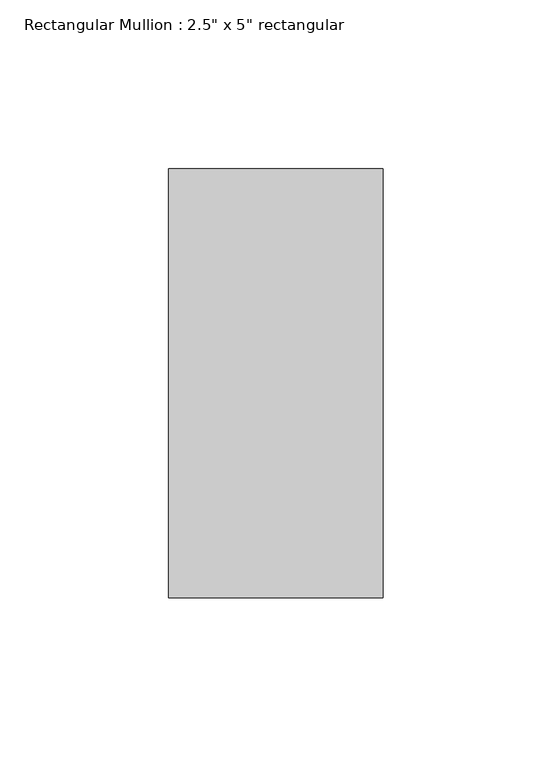
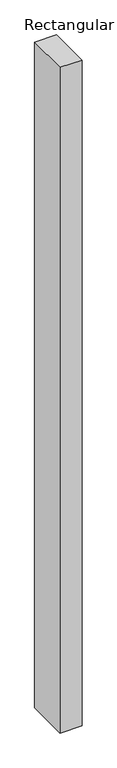
"""IFC4 building model written with IfcOpenShell, lengths in millimetres: member geometry."""

from ifc_helpers import new_model, si_unit, frame, origin, place, context, project, spatial, polyline, outline, extrude, source, transform, mapped, element, save


def member_003cbd34(model_context):
    return source(origin(), model_context, "Body", "SweptSolid", [
        extrude(outline(polyline([(0.0, 63.5), (0.0, -63.5), (-63.5, -63.5), (-63.5, 63.5), (0.0, 63.5)])), frame((0.0, 0.0, -2036.2333333), z_axis=(0.0, 0.0, 1.0), x_axis=(1.0, 0.0, 0.0)), (0.0, 0.0, 1.0), 2036.2333333),
    ])


if __name__ == "__main__":
    model = new_model("IFC4")
    model_context = context("Model", 3, world=origin())
    ifc_project = project(units=[si_unit("LENGTHUNIT", "METRE", prefix="MILLI")], contexts=[model_context])
    site = spatial("IfcSite", under=ifc_project)
    building = spatial("IfcBuilding", under=site)
    placement = place(None, origin())
    member_shape = member_003cbd34(model_context)
    element("IfcMember", 1, ObjectType="Rectangular Mullion : 2.5\" x 5\" rectangular", at=placement, inside=building, context=model_context, shape_type="MappedRepresentation", body=[
        mapped(member_shape, transform((0.0, 0.0, 0.0), x_axis=(1.0, 0.0, 0.0), y_axis=(0.0, 1.0, 0.0), z_axis=(0.0, 0.0, 1.0))),
    ])
    save(model, "model.ifc")

# Revit data of these elements
# Type "Rectangular Mullion : 2.5\" x 5\" rectangular"
#   built-in parameter 1007304 = 0.416667 (stored number, unit not read)
#   built-in parameter 1007301 = 0.104167 (stored number, unit not read)
#   built-in parameter 1007300 = 0.104167 (stored number, unit not read)
# Element 1 (IfcMember, "Rectangular Mullion : 2.5\" x 5\" rectangular")
#   Materials on its faces: "Aluminum"
# Materials
#   "Aluminum": class "Metal", colour RGB 247 247 247, transparency 0, Description = "Aluminum 6061", Cost = 0
